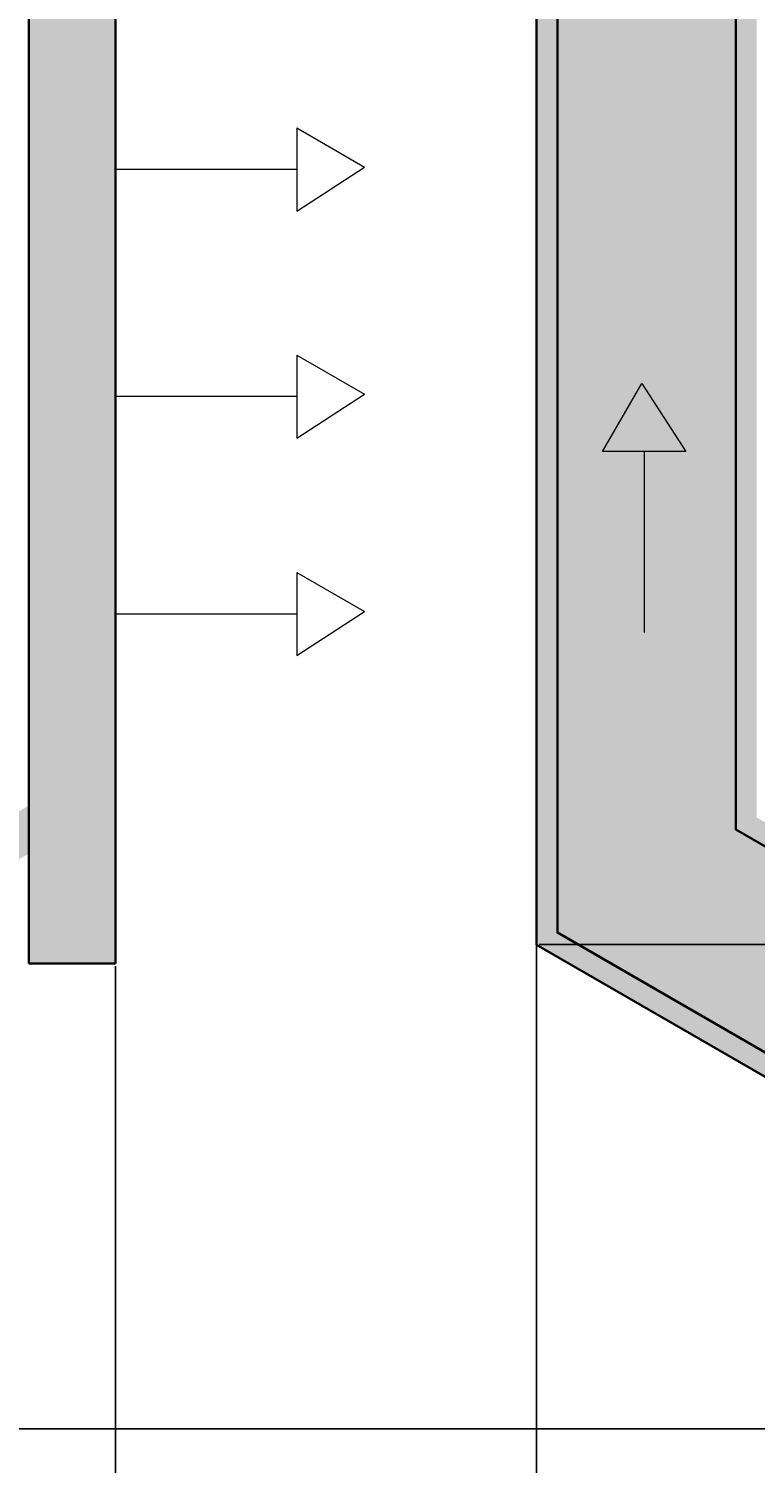
# Model space of a CAD drawing. Units: inches. Extents: x -1 to 292, y -3 to 199.
# Tile 39 of 52: x 203 to 220, y 43 to 77. Entities that reach past the tile are written whole.
import ezdxf

# ---------------------------------------------------------------- set-up
doc = ezdxf.new("R2010")
doc.units = ezdxf.units.IN
doc.header["$MEASUREMENT"] = 0
for name, color, linetype, lineweight in [('M-ANNO-SYMB', 1, 'Continuous', 18), ('M-DIMS', 2, 'Continuous', 18), ('M-EQPM', 7, 'Continuous', 35), ('M-PATT', 8, 'Continuous', 13)]:
    doc.layers.add(name, color=color, linetype=linetype, lineweight=lineweight)
doc.styles.get("Standard").update_dxf_attribs({"font": 'arial.ttf'})
doc.dimstyles.get("Standard").update_dxf_attribs({"dimtxt": 0.18, "dimasz": 0.18, "dimexe": 0.18, "dimexo": 0.0625, "dimgap": 0.09, "dimtad": 0, "dimtih": 1, "dimtoh": 1, "dimdec": 4, "dimzin": 0, "dimdsep": 46, "dimtxsty": 'Standard', "dimcen": 0.09, "dimadec": 0, "dimazin": 0, "dimtfac": 1, "dimtdec": 4, "dimtofl": 0, "dimtmove": 0, "dimatfit": 3, "dimfxl": 1, "dimtolj": 1, "dimtzin": 0, "dimarcsym": 0})

# ---------------------------------------------------------------- blocks, each defined once
blk = doc.blocks.new('FLOW-ARROW-GAS')
for p, q in [((201.507, 38.14), (201.507, 36.14)), ((201.507, 38.14), (203.137, 37.199)), ((201.507, 37.14), (197.151, 37.14)), ((201.507, 36.14), (203.137, 37.199))]:
    blk.add_line(p, q)
blk = doc.blocks.new('FLOW-ARROW-WATER')
blk.add_line((223.29, 53.741), (227.063, 51.564))
blk.add_lwpolyline([(222.79, 52.875), (221.849, 54.506), (223.79, 54.608)], close=True)
blk = doc.blocks.new('DUCT-FLANGE')
for p, q in [((0, 34), (0, 0)), ((0, 34), (2.089, 34)), ((2.089, 34), (2.089, 0)), ((0, 0), (2.089, 0))]:
    blk.add_line(p, q)
blk = doc.blocks.new('*D7')
at = {"layer": 'Defpoints', "color": 0, "transparency": 16777216}
for p in [(21.861, 54.582), (205.115, 54.582), (21.861, 39.982)]:
    blk.add_point(p, dxfattribs=at)
at = {"layer": 'M-DIMS', "color": 0, "lineweight": -2, "transparency": 16777216}
for p, q in [((21.861, 54.52), (21.861, 39.802)), ((205.115, 54.52), (205.115, 39.802)), ((22.041, 39.982), (113.033, 39.982)), ((204.935, 39.982), (113.944, 39.982))]:
    blk.add_line(p, q, dxfattribs=at)
at = {"layer": 'M-DIMS', "color": 0, "transparency": 16777216}
for points in [[(22.041, 40.012), (22.041, 39.952), (21.861, 39.982)], [(204.935, 40.012), (204.935, 39.952), (205.115, 39.982)]]:
    blk.add_solid(points, dxfattribs=at)
at = {"layer": 'M-DIMS', "color": 0, "transparency": 16777216, "insert": (113.488, 39.982), "char_height": 0.18, "attachment_point": 5}
blk.add_mtext('\\A1;183.25', dxfattribs=at)
blk = doc.blocks.new('*D10')
at = {"layer": 'Defpoints', "color": 0, "transparency": 16777216}
for p in [(169.176, 99.774), (169.176, 43.391), (292.04, 43.391)]:
    blk.add_point(p, dxfattribs=at)
at = {"layer": 'M-DIMS', "color": 0, "lineweight": -2, "transparency": 16777216}
for p, q in [((169.239, 99.774), (292.22, 99.774)), ((292.04, 99.594), (292.04, 71.764)), ((292.04, 43.571), (292.04, 71.4)), ((169.239, 43.391), (292.22, 43.391))]:
    blk.add_line(p, q, dxfattribs=at)
at = {"layer": 'M-DIMS', "color": 0, "transparency": 16777216}
for points in [[(292.01, 99.594), (292.07, 99.594), (292.04, 99.774)], [(292.01, 43.571), (292.07, 43.571), (292.04, 43.391)]]:
    blk.add_solid(points, dxfattribs=at)
at = {"layer": 'M-DIMS', "color": 0, "transparency": 16777216, "insert": (292.04, 71.582), "char_height": 0.18, "attachment_point": 5}
blk.add_mtext('\\A1;56.38', dxfattribs=at)
blk = doc.blocks.new('*D24')
at = {"layer": 'Defpoints', "color": 0, "transparency": 16777216}
for p in [(215.241, 55.034), (205.115, 54.582), (215.241, -2.71)]:
    blk.add_point(p, dxfattribs=at)
at = {"layer": 'M-DIMS', "color": 0, "lineweight": -2, "transparency": 16777216}
for p, q in [((215.241, 54.971), (215.241, -2.89)), ((205.115, 54.52), (205.115, -2.89)), ((205.295, -2.71), (209.722, -2.71)), ((215.061, -2.71), (210.634, -2.71))]:
    blk.add_line(p, q, dxfattribs=at)
at = {"layer": 'M-DIMS', "color": 0, "transparency": 16777216}
for points in [[(205.295, -2.68), (205.295, -2.74), (205.115, -2.71)], [(215.061, -2.68), (215.061, -2.74), (215.241, -2.71)]]:
    blk.add_solid(points, dxfattribs=at)
at = {"layer": 'M-DIMS', "color": 0, "transparency": 16777216, "insert": (210.178, -2.71), "char_height": 0.18, "attachment_point": 5}
blk.add_mtext('\\A1;10.125', dxfattribs=at)
blk = doc.blocks.new('*D25')
at = {"layer": 'Defpoints', "color": 0, "transparency": 16777216}
for p in [(273.066, 88.419), (215.241, 88.13), (273.066, -2.71)]:
    blk.add_point(p, dxfattribs=at)
at = {"layer": 'M-DIMS', "color": 0, "lineweight": -2, "transparency": 16777216}
for p, q in [((273.066, 88.357), (273.066, -2.89)), ((215.241, 88.068), (215.241, -2.89)), ((215.421, -2.71), (243.76, -2.71)), ((272.886, -2.71), (244.547, -2.71))]:
    blk.add_line(p, q, dxfattribs=at)
at = {"layer": 'M-DIMS', "color": 0, "transparency": 16777216}
for points in [[(215.421, -2.68), (215.421, -2.74), (215.241, -2.71)], [(272.886, -2.68), (272.886, -2.74), (273.066, -2.71)]]:
    blk.add_solid(points, dxfattribs=at)
at = {"layer": 'M-DIMS', "color": 0, "transparency": 16777216, "insert": (244.153, -2.71), "char_height": 0.18, "attachment_point": 5}
blk.add_mtext('\\A1;57.83', dxfattribs=at)
blk = doc.blocks.new('*D26')
at = {"layer": 'Defpoints', "color": 0, "transparency": 16777216}
for p in [(215.241, 88.13), (215.241, 55.034), (229.841, 55.034)]:
    blk.add_point(p, dxfattribs=at)
at = {"layer": 'M-DIMS', "color": 0, "lineweight": -2, "transparency": 16777216}
for p, q in [((215.303, 88.13), (230.021, 88.13)), ((229.841, 87.95), (229.841, 71.764)), ((229.841, 55.214), (229.841, 71.4)), ((215.303, 55.034), (230.021, 55.034))]:
    blk.add_line(p, q, dxfattribs=at)
at = {"layer": 'M-DIMS', "color": 0, "transparency": 16777216}
for points in [[(229.811, 87.95), (229.871, 87.95), (229.841, 88.13)], [(229.811, 55.214), (229.871, 55.214), (229.841, 55.034)]]:
    blk.add_solid(points, dxfattribs=at)
at = {"layer": 'M-DIMS', "color": 0, "transparency": 16777216, "insert": (229.841, 71.582), "char_height": 0.18, "attachment_point": 5}
blk.add_mtext('\\A1;33.1', dxfattribs=at)

msp = doc.modelspace()

# ---------------------------------------------------------------- hatches: boundary and pattern name
at = {"layer": 'M-PATT'}
h = msp.add_hatch(color=256, dxfattribs=at)
h.set_gradient(color1=(0, 255, 255), color2=(0, 255, 255), tint=1, name='CYLINDER')
h.paths.add_polyline_path([(256.8092, 99.5764), (256.4077, 99.3157), (253.7155, 100.87), (251.3221, 99.3157), (248.6299, 100.87), (246.2365, 99.3157), (243.5443, 100.87), (241.1509, 99.3157), (238.4587, 100.87), (236.4209, 99.5466), (236.4209, 97.1861), (234.9209, 97.1861), (234.9209, 99.9764), (233.3731, 100.87), (230.9797, 99.3157, 1.0704128)])
h.paths.add_polyline_path([(234.4549, 44.5975, 1), (253.3518, 44.5975, 1)])
h.paths.add_polyline_path([(235.4822, 48.8821), (220.034, 57.8011), (220.034, 85.363), (232.4507, 92.5318, -0.0853739), (231.0925, 96.7051), (215.7407, 87.8418), (215.7407, 55.3224), (234.4552, 44.5176, -0.0021162), (234.4549, 44.5975, -0.1182098)])
h.paths.add_polyline_path([(222.7904, 52.8755), (221.8492, 54.5058), (223.7904, 54.6075)], flags=16)
h.paths.add_polyline_path([(216.828, 66.8912), (217.7692, 68.5216), (218.828, 66.8912)], flags=16)
h.paths.add_polyline_path([(216.8084, 83.826), (217.7497, 85.4564), (218.8084, 83.826)], flags=16)
h.paths.add_polyline_path([(226.468, 92.8803), (228.3442, 93.0348), (227.6068, 91.2362)], flags=16)
h.paths.add_polyline_path([(272.5659, 88.1304), (260.2765, 95.2257), (259.0113, 93.0196), (263.0639, 91.1046), (263.4912, 92.0087), (264.5631, 90.4612), (262.6367, 90.2004), (263.0639, 91.1046), (259.0113, 93.0196), (257.8918, 91.0677), (267.7726, 85.363), (267.7726, 57.8011), (255.5043, 50.718), (257.0663, 46.085), (272.5659, 55.0337)])
h.paths.add_polyline_path([(263.6286, 51.5636), (261.7461, 51.5636), (262.6286, 53.2956)], flags=16)
h.paths.add_polyline_path([(269.8773, 65.3608), (268.8186, 66.9911), (270.8186, 66.9911)], flags=16)
h.paths.add_polyline_path([(269.8773, 80.8843), (268.8186, 82.5146), (270.8186, 82.5146)], flags=16)
h.paths.add_polyline_path([(255.5043, 50.718), (252.3244, 48.8821, -0.1182098), (253.3518, 44.5975, -0.0177685), (253.3279, 43.9266), (257.0663, 46.085)])
h.paths.add_polyline_path([(260.2765, 95.2257), (256.7809, 97.2439, -0.0959457), (255.356, 92.5318), (257.8918, 91.0677)])
h = msp.add_hatch(color=256, dxfattribs=at)
h.set_gradient(color1=(76, 38, 47), color2=(76, 38, 47), tint=1, name='CYLINDER')
h.paths.add_polyline_path([(267.2726, 58.0898), (255.3414, 51.2013), (255.5043, 50.718), (267.7726, 57.8011), (267.7726, 85.363), (257.8918, 91.0677), (257.643, 90.634), (267.2726, 85.0743)])
h.paths.add_polyline_path([(272.5659, 55.0337), (257.0663, 46.085), (257.2293, 45.6017), (273.0659, 54.745), (273.0659, 88.4191), (260.5253, 95.6595), (260.2765, 95.2257), (272.5659, 88.1304)])
h.paths.add_polyline_path([(215.2407, 55.0337), (234.4787, 43.9266, -0.0156517), (234.4552, 44.5176), (215.7407, 55.3224), (215.7407, 87.8418), (231.0925, 96.7051, -0.0104859), (231.0257, 97.2439), (215.2407, 88.1304)])
h.paths.add_polyline_path([(220.034, 57.8011), (235.4822, 48.8821, -0.0132367), (235.7207, 49.3218), (220.534, 58.0898), (220.534, 85.0743), (232.6923, 92.0939, -0.0096587), (232.4507, 92.5318), (220.034, 85.363)])
h = msp.add_hatch(color=256, dxfattribs=at)
h.set_gradient(color1=(76, 38, 47), color2=(76, 38, 47), tint=1, name='CYLINDER')
h.paths.add_polyline_path([(40.8628, 91.6478), (40.3591, 92.5203), (23.9502, 85.5552), (23.9502, 84.4688)])
h.paths.add_polyline_path([(52.8586, 93.6403), (42.9977, 93.6403), (40.3591, 92.5203), (40.8628, 91.6478), (43.2011, 92.6403), (54.4604, 92.6403, -0.0601508)])
h.paths.add_polyline_path([(23.9502, 88.5821), (21.8612, 88.5821), (21.8612, 54.5821), (23.9502, 54.5821)])
h.paths.add_polyline_path([(23.9502, 58.376), (23.9502, 57.2213), (42.9332, 46.2615), (50.4659, 46.2615, -0.0351813), (50.9409, 47.2615), (43.2011, 47.2615)])
h.paths.add_polyline_path([(179.5897, 93.6403), (174.1181, 93.6403, -0.0601508), (172.5163, 92.6403), (179.5897, 92.6403)])
h.paths.add_polyline_path([(183.979, 93.6403), (181.5897, 93.6403), (181.5897, 92.6403), (183.7755, 92.6403), (203.0265, 84.4688), (203.0265, 85.5552)])
h.paths.add_polyline_path([(205.1155, 88.5821), (203.0265, 88.5821), (203.0265, 54.5821), (205.1155, 54.5821)])
h.paths.add_polyline_path([(203.0265, 57.2213), (203.0265, 58.376), (183.7755, 47.2615), (181.5897, 47.2615), (181.5897, 46.2615), (184.0435, 46.2615)])
h.paths.add_polyline_path([(179.5897, 47.2615), (176.0358, 47.2615, -0.0351813), (176.5107, 46.2615), (179.5897, 46.2615)])
h = msp.add_hatch(color=256, dxfattribs=at)
h.set_gradient(color1=(0, 0, 255), color2=(0, 0, 255), tint=1, name='CYLINDER')
h.paths.add_polyline_path([(227.6068, 91.2362), (228.3442, 93.0348), (226.468, 92.8803)])
h.paths.add_polyline_path([(218.8084, 83.826), (217.7497, 85.4564), (216.8084, 83.826)])
h.paths.add_polyline_path([(262.6367, 90.2004), (264.5631, 90.4612), (263.4912, 92.0087)])
h.paths.add_polyline_path([(217.7692, 68.5216), (216.828, 66.8912), (218.828, 66.8912)])
h.paths.add_polyline_path([(223.7904, 54.6075), (221.8492, 54.5058), (222.7904, 52.8755)])
h.paths.add_polyline_path([(262.6286, 53.2956), (261.7461, 51.5636), (263.6286, 51.5636)])
h.paths.add_polyline_path([(268.8186, 82.5146), (269.8773, 80.8843), (270.8186, 82.5146)])
h.paths.add_polyline_path([(268.8186, 66.9911), (269.8773, 65.3608), (270.8186, 66.9911)])

# ---------------------------------------------------------------- linework, layer by layer
at = {"layer": 'M-EQPM'}
for points in [[(231.0257, 97.2439), (215.2407, 88.1304), (215.2407, 55.0337), (234.4787, 43.9266)], [(231.0925, 96.7051), (215.7407, 87.8418), (215.7407, 55.3224), (234.4552, 44.5176)], [(232.4507, 92.5318), (220.034, 85.363), (220.034, 57.8011), (235.4822, 48.8821)]]:
    msp.add_lwpolyline(points, dxfattribs=at)

# ---------------------------------------------------------------- block references
at = {"layer": 'M-ANNO-SYMB'}
for p in [(7.9644, 36.5298), (7.9644, 31.0696), (7.9644, 25.8419)]:
    msp.add_blockref('FLOW-ARROW-GAS', p, dxfattribs=at)
at = {"layer": 'M-ANNO-SYMB', "rotation": 300.0000000000012}
msp.add_blockref('FLOW-ARROW-WATER', (59.6413, 233.3957), dxfattribs=at)
at = {"layer": 'M-EQPM'}
msp.add_blockref('DUCT-FLANGE', (203.0263, 54.582), dxfattribs=at)

# ---------------------------------------------------------------- dimensions: what is measured, and where the dimension line sits
at = {"layer": 'M-DIMS'}
for base, p1, p2, angle, override, picture, middle in [((292.0399, 43.3906), (169.176, 99.7735), (169.176, 43.3906), 90, {"dimdec": 2, "dimlfac": 1, "dimrnd": 0, "dimzin": 0, "dimdsep": 46, "dimlunit": 2}, '*D10', (292.0399, 71.5821)), ((229.8407, 55.0337), (215.2407, 88.1304), (215.2407, 55.0337), 270, {"dimdec": 1, "dimlfac": 1, "dimrnd": 0, "dimzin": 0, "dimdsep": 46, "dimlunit": 2}, '*D26', (229.8407, 71.5821)), ((21.8612, 39.9821), (205.1155, 54.5821), (21.8612, 54.5821), 180, {"dimdec": 2, "dimlfac": 1, "dimrnd": 0, "dimzin": 0, "dimdsep": 46, "dimlunit": 2}, '*D7', (113.4883, 39.9821))]:
    dim = msp.add_linear_dim(base=base, p1=p1, p2=p2, angle=angle, dimstyle='Standard', override=override, dxfattribs=at)
    dim.commit()
    dim.dimension.update_dxf_attribs({"geometry": picture, "text_midpoint": middle})
for base, p1, p2, override, picture, middle in [((273.0659, -2.7104), (215.2407, 88.1304), (273.0659, 88.4191), {"dimdec": 2, "dimlfac": 1, "dimrnd": 0, "dimzin": 0, "dimdsep": 46, "dimlunit": 2}, '*D25', (244.1533, -2.7104)), ((215.2407, -2.7104), (205.1155, 54.5821), (215.2407, 55.0337), {"dimdec": 3, "dimlfac": 1, "dimrnd": 0, "dimzin": 0, "dimdsep": 46, "dimlunit": 2}, '*D24', (210.1781, -2.7104))]:
    dim = msp.add_linear_dim(base=base, p1=p1, p2=p2, dimstyle='Standard', override=override, dxfattribs=at)
    dim.commit()
    dim.dimension.update_dxf_attribs({"geometry": picture, "text_midpoint": middle})

doc.saveas('drawing.dxf')
